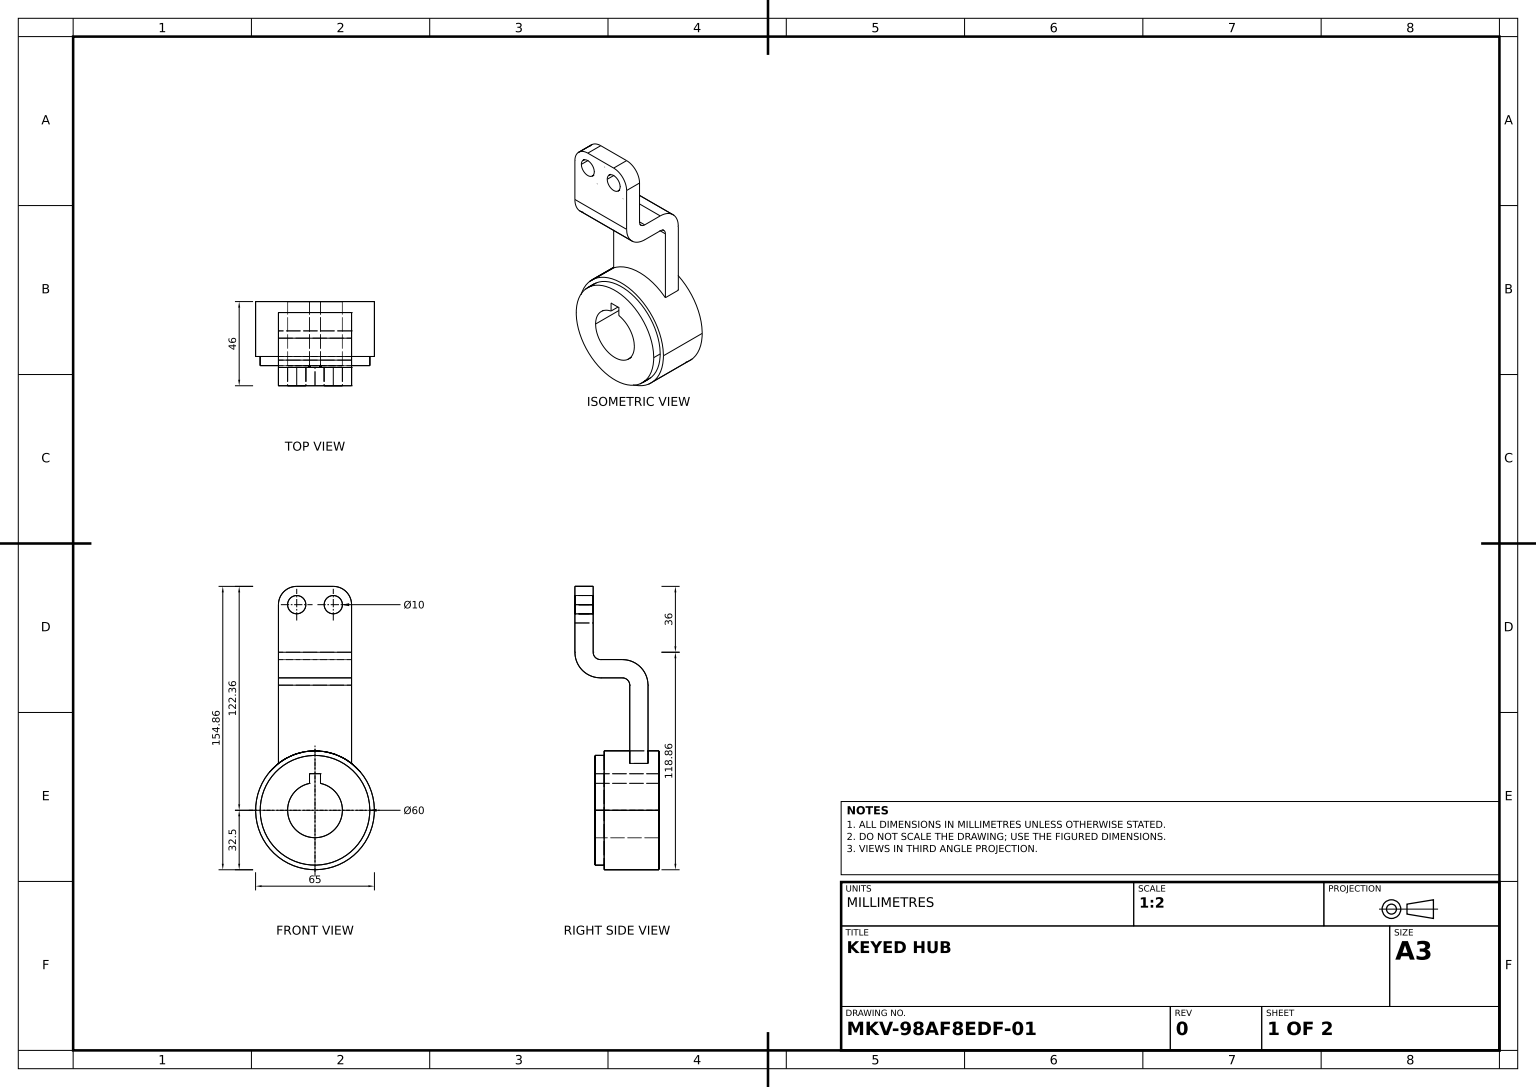
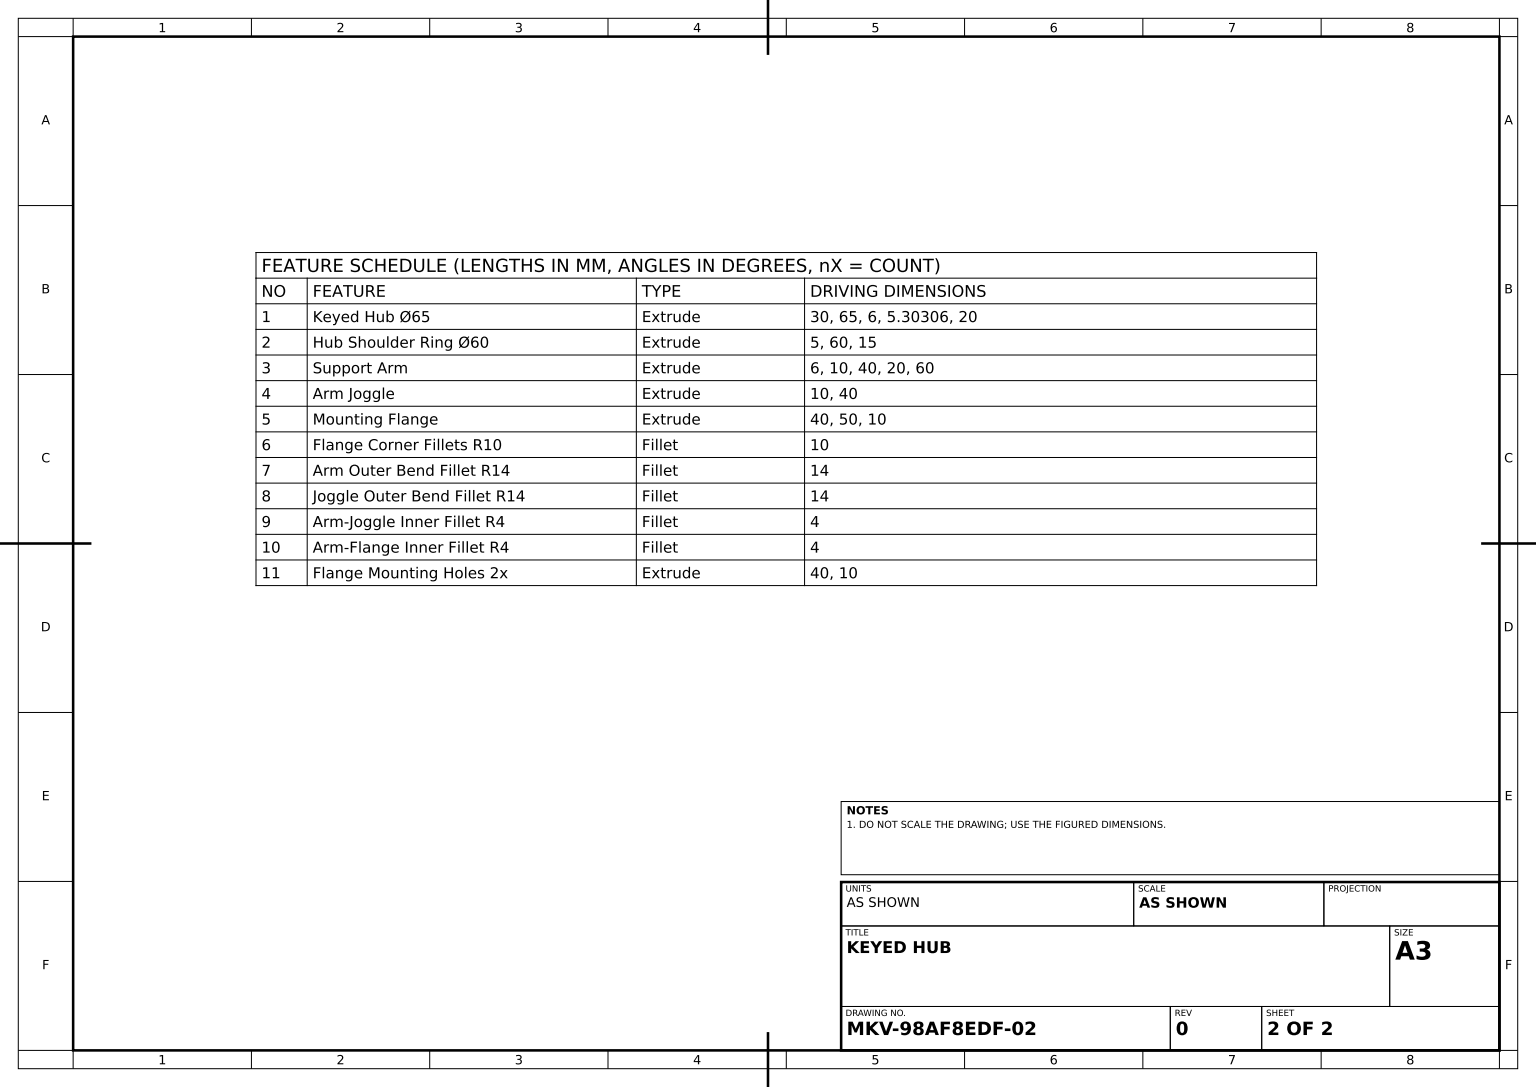
from build123d import *

# Parameters (mm, degrees)
KEYED_HUB_PROFILE_R             = 32.5
KEYED_HUB_65_DEPTH              = 30
HUB_SHOULDER_PROFILE_R          = 30
HUB_SHOULDER_RING_60_DEPTH      = 5
SUPPORT_ARM_PROFILE_W           = 40
SUPPORT_ARM_PROFILE_H           = 60
SUPPORT_ARM_DEPTH               = 10
ARM_JOGGLE_PROFILE_W            = 40
ARM_JOGGLE_PROFILE_H            = 40
ARM_JOGGLE_DEPTH                = 10
MOUNTING_FLANGE_PROFILE_W       = 10
MOUNTING_FLANGE_PROFILE_H       = 50
MOUNTING_FLANGE_DEPTH           = 40
FLANGE_CORNER_FILLETS_R10_R     = 10
ARM_OUTER_BEND_FILLET_R14_R     = 14
JOGGLE_OUTER_BEND_FILLET_R14_R  = 14
ARM_JOGGLE_INNER_FILLET_R4_R    = 4
ARM_FLANGE_INNER_FILLET_R4_R    = 4
FLANGE_MOUNTING_HOLES_PROFILE_R = 5
FLANGE_MOUNTING_HOLES_2X_DEPTH  = 40


with BuildPart() as part:
    # Keyed Hub Profile → Keyed Hub Ø65 (new body)
    with BuildSketch(Plane.XY):
        Circle(KEYED_HUB_PROFILE_R)
        with BuildLine():
            Line((-3, 20), (3, 20))
            Line((3, 20), (3, 14.696938457))
            ThreePointArc((3, 14.696938457), (0, -15), (-3, 14.696938457))
            Line((-3, 14.696938457), (-3, 20))
        make_face(mode=Mode.SUBTRACT)
    extrude(amount=KEYED_HUB_65_DEPTH)

    # Hub Shoulder Profile → Hub Shoulder Ring Ø60 (add)
    with BuildSketch(Plane.XY.offset(30)):
        Circle(HUB_SHOULDER_PROFILE_R)
        with BuildLine():
            Line((-3, 14.696938457), (-3, 20))
            Line((-3, 20), (3, 20))
            Line((3, 20), (3, 14.696938457))
            ThreePointArc((3, 14.696938457), (0, -15), (-3, 14.696938457))
        make_face(mode=Mode.SUBTRACT)
    extrude(amount=HUB_SHOULDER_RING_60_DEPTH)

    # Support Arm Profile → Support Arm (add)
    with BuildSketch(Plane.XY.offset(6)):
        with Locations((0, 52.360679775)):
            Rectangle(SUPPORT_ARM_PROFILE_W, SUPPORT_ARM_PROFILE_H)
    extrude(amount=SUPPORT_ARM_DEPTH)

    # Arm Joggle Profile → Arm Joggle (add)
    with BuildSketch(Plane(origin=(0, 82.360679775, 0), x_dir=(1, 0, 0), z_dir=(0, 1, 0))):
        with Locations((0, -26)):
            Rectangle(ARM_JOGGLE_PROFILE_W, ARM_JOGGLE_PROFILE_H)
    extrude(amount=-ARM_JOGGLE_DEPTH)

    # Mounting Flange Profile → Mounting Flange (add)
    with BuildSketch(Plane(origin=(20, 0, 0), x_dir=(0, 0, -1), z_dir=(1, 0, 0))):
        with Locations((-41, 97.360679775)):
            Rectangle(MOUNTING_FLANGE_PROFILE_W, MOUNTING_FLANGE_PROFILE_H)
    extrude(amount=-MOUNTING_FLANGE_DEPTH)

    # Flange Corner Fillets R10
    flange_corner_fillets_r10_edges = [part.edges().sort_by_distance(p)[0] for p in [
        (20, 122.360679775, 41),
        (-20, 122.360679775, 41),
    ]]
    fillet(flange_corner_fillets_r10_edges, radius=FLANGE_CORNER_FILLETS_R10_R)

    # Arm Outer Bend Fillet R14
    arm_outer_bend_fillet_r14_edges = [part.edges().sort_by_distance(p)[0] for p in [
        (0, 82.360679775, 6),
    ]]
    fillet(arm_outer_bend_fillet_r14_edges, radius=ARM_OUTER_BEND_FILLET_R14_R)

    # Joggle Outer Bend Fillet R14
    joggle_outer_bend_fillet_r14_edges = [part.edges().sort_by_distance(p)[0] for p in [
        (0, 72.360679775, 46),
    ]]
    fillet(joggle_outer_bend_fillet_r14_edges, radius=JOGGLE_OUTER_BEND_FILLET_R14_R)

    # Arm-Joggle Inner Fillet R4
    arm_joggle_inner_fillet_r4_edges = [part.edges().sort_by_distance(p)[0] for p in [
        (0, 72.360679775, 16),
    ]]
    fillet(arm_joggle_inner_fillet_r4_edges, radius=ARM_JOGGLE_INNER_FILLET_R4_R)

    # Arm-Flange Inner Fillet R4
    arm_flange_inner_fillet_r4_edges = [part.edges().sort_by_distance(p)[0] for p in [
        (0, 82.360679775, 36),
    ]]
    fillet(arm_flange_inner_fillet_r4_edges, radius=ARM_FLANGE_INNER_FILLET_R4_R)

    # Flange Mounting Holes Profile → Flange Mounting Holes 2x (cut)
    with BuildSketch(Plane.XY.offset(46)):
        with Locations((-10, 112.360679775)):
            Circle(FLANGE_MOUNTING_HOLES_PROFILE_R)
        with Locations((10, 112.360679775)):
            Circle(FLANGE_MOUNTING_HOLES_PROFILE_R)
    extrude(amount=-FLANGE_MOUNTING_HOLES_2X_DEPTH, mode=Mode.SUBTRACT)


solid = part.part
